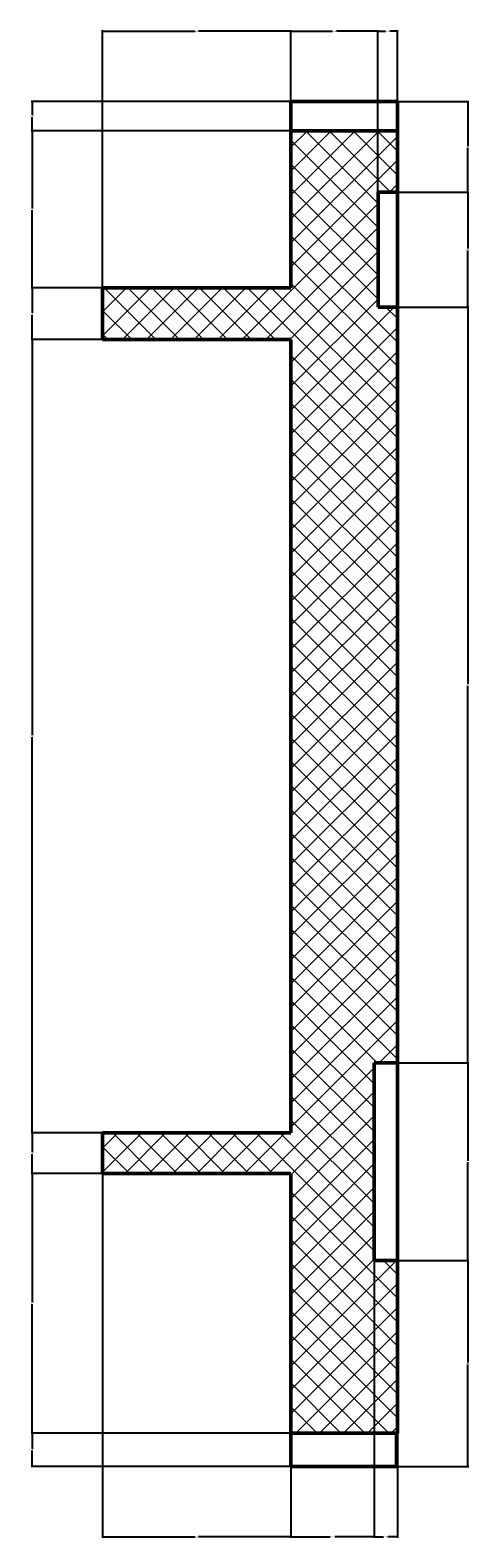
# Model space of a CAD drawing. Units: millimetres. Extents: x 2637 to 3282, y 1554 to 2264.
# Tile 3 of 3: x 3199 to 3282, y 1976 to 2260. Entities that reach past the tile are written whole.
import ezdxf

# ---------------------------------------------------------------- set-up
doc = ezdxf.new("R2010")
doc.units = ezdxf.units.MM
for name, color, linetype, lineweight in [('M-DIMS', 2, 'Continuous', 18), ('M-HATC', 8, 'Continuous', 18), ('M-OUTL', 7, 'Continuous', 50)]:
    doc.layers.add(name, color=color, linetype=linetype, lineweight=lineweight)
doc.styles.get("Standard").update_dxf_attribs({"font": 'arial.ttf'})
doc.dimstyles.get("Standard").update_dxf_attribs({"dimtxt": 0.18, "dimasz": 0.18, "dimexe": 0.18, "dimexo": 0.0625, "dimgap": 0.09, "dimtad": 0, "dimtih": 1, "dimtoh": 1, "dimdec": 4, "dimzin": 0, "dimdsep": 46, "dimtxsty": 'Standard', "dimcen": 0.09, "dimadec": 0, "dimazin": 0, "dimtfac": 1, "dimtdec": 4, "dimtofl": 0, "dimtmove": 0, "dimatfit": 3, "dimfxl": 1, "dimtolj": 1, "dimtzin": 0, "dimarcsym": 0})

# ---------------------------------------------------------------- blocks, each defined once
blk = doc.blocks.new('*D25')
at = {"layer": 'Defpoints', "color": 0, "transparency": 16777216}
for p in [(3247.95, 2259.5), (3212.55, 2211.25), (3247.95, 2211.25)]:
    blk.add_point(p, dxfattribs=at)
at = {"layer": 'M-DIMS', "color": 0, "lineweight": -2, "transparency": 16777216}
for p, q in [((3212.55, 2211.32), (3212.55, 2259.68)), ((3212.73, 2259.5), (3229.93, 2259.5)), ((3247.77, 2259.5), (3230.58, 2259.5)), ((3247.95, 2211.32), (3247.95, 2259.68))]:
    blk.add_line(p, q, dxfattribs=at)
at = {"layer": 'M-DIMS', "color": 0, "transparency": 16777216}
for points in [[(3212.73, 2259.53), (3212.73, 2259.47), (3212.55, 2259.5)], [(3247.77, 2259.53), (3247.77, 2259.47), (3247.95, 2259.5)]]:
    blk.add_solid(points, dxfattribs=at)
at = {"layer": 'M-DIMS', "color": 0, "transparency": 16777216, "insert": (3230.25, 2259.5), "char_height": 0.18, "attachment_point": 5}
blk.add_mtext('\\A1;35.4', dxfattribs=at)
blk = doc.blocks.new('*D26')
at = {"layer": 'Defpoints', "color": 0, "transparency": 16777216}
for p in [(3264.31, 2259.5), (3247.95, 2246.25), (3264.31, 2229.26)]:
    blk.add_point(p, dxfattribs=at)
at = {"layer": 'M-DIMS', "color": 0, "lineweight": -2, "transparency": 16777216}
for p, q in [((3247.95, 2246.31), (3247.95, 2259.68)), ((3248.13, 2259.5), (3255.75, 2259.5)), ((3264.13, 2259.5), (3256.52, 2259.5)), ((3264.31, 2229.32), (3264.31, 2259.68))]:
    blk.add_line(p, q, dxfattribs=at)
at = {"layer": 'M-DIMS', "color": 0, "transparency": 16777216}
for points in [[(3248.13, 2259.53), (3248.13, 2259.47), (3247.95, 2259.5)], [(3264.13, 2259.53), (3264.13, 2259.47), (3264.31, 2259.5)]]:
    blk.add_solid(points, dxfattribs=at)
at = {"layer": 'M-DIMS', "color": 0, "transparency": 16777216, "insert": (3256.13, 2259.5), "char_height": 0.18, "attachment_point": 5}
blk.add_mtext('\\A1;16.36', dxfattribs=at)
blk = doc.blocks.new('*D27')
at = {"layer": 'Defpoints', "color": 0, "transparency": 16777216}
for p in [(3267.95, 2259.5), (3264.31, 2229.26), (3267.95, 2229.26)]:
    blk.add_point(p, dxfattribs=at)
at = {"layer": 'M-DIMS', "color": 0, "lineweight": -2, "transparency": 16777216}
for p, q in [((3264.31, 2229.32), (3264.31, 2259.68)), ((3264.49, 2259.5), (3265.74, 2259.5)), ((3267.77, 2259.5), (3266.53, 2259.5)), ((3267.95, 2229.32), (3267.95, 2259.68))]:
    blk.add_line(p, q, dxfattribs=at)
at = {"layer": 'M-DIMS', "color": 0, "transparency": 16777216}
for points in [[(3264.49, 2259.53), (3264.49, 2259.47), (3264.31, 2259.5)], [(3267.77, 2259.53), (3267.77, 2259.47), (3267.95, 2259.5)]]:
    blk.add_solid(points, dxfattribs=at)
at = {"layer": 'M-DIMS', "color": 0, "transparency": 16777216, "insert": (3266.13, 2259.5), "char_height": 0.18, "attachment_point": 5}
blk.add_mtext('\\A1;3.639', dxfattribs=at)
blk = doc.blocks.new('*D28')
at = {"layer": 'Defpoints', "color": 0, "transparency": 16777216}
for p in [(3212.55, 2044.85), (3247.95, 2044.85), (3247.95, 1976.59)]:
    blk.add_point(p, dxfattribs=at)
at = {"layer": 'M-DIMS', "color": 0, "lineweight": -2, "transparency": 16777216}
for p, q in [((3212.55, 2044.79), (3212.55, 1976.41)), ((3247.95, 2044.79), (3247.95, 1976.41)), ((3212.73, 1976.59), (3229.93, 1976.59)), ((3247.77, 1976.59), (3230.58, 1976.59))]:
    blk.add_line(p, q, dxfattribs=at)
at = {"layer": 'M-DIMS', "color": 0, "transparency": 16777216}
for points in [[(3212.73, 1976.62), (3212.73, 1976.56), (3212.55, 1976.59)], [(3247.77, 1976.62), (3247.77, 1976.56), (3247.95, 1976.59)]]:
    blk.add_solid(points, dxfattribs=at)
at = {"layer": 'M-DIMS', "color": 0, "transparency": 16777216, "insert": (3230.25, 1976.59), "char_height": 0.18, "attachment_point": 5}
blk.add_mtext('\\A1;35.4', dxfattribs=at)
blk = doc.blocks.new('*D29')
at = {"layer": 'Defpoints', "color": 0, "transparency": 16777216}
for p in [(3263.56, 2028.52), (3247.95, 1989.84), (3263.56, 1976.59)]:
    blk.add_point(p, dxfattribs=at)
at = {"layer": 'M-DIMS', "color": 0, "lineweight": -2, "transparency": 16777216}
for p, q in [((3263.56, 2028.46), (3263.56, 1976.41)), ((3247.95, 1989.77), (3247.95, 1976.41)), ((3248.13, 1976.59), (3255.3, 1976.59)), ((3263.38, 1976.59), (3256.21, 1976.59))]:
    blk.add_line(p, q, dxfattribs=at)
at = {"layer": 'M-DIMS', "color": 0, "transparency": 16777216}
for points in [[(3248.13, 1976.62), (3248.13, 1976.56), (3247.95, 1976.59)], [(3263.38, 1976.62), (3263.38, 1976.56), (3263.56, 1976.59)]]:
    blk.add_solid(points, dxfattribs=at)
at = {"layer": 'M-DIMS', "color": 0, "transparency": 16777216, "insert": (3255.76, 1976.59), "char_height": 0.18, "attachment_point": 5}
blk.add_mtext('\\A1;15.612', dxfattribs=at)
blk = doc.blocks.new('*D30')
at = {"layer": 'Defpoints', "color": 0, "transparency": 16777216}
for p in [(3263.56, 2028.52), (3267.95, 2028.52), (3267.95, 1976.59)]:
    blk.add_point(p, dxfattribs=at)
at = {"layer": 'M-DIMS', "color": 0, "lineweight": -2, "transparency": 16777216}
for p, q in [((3263.56, 2028.46), (3263.56, 1976.41)), ((3267.95, 2028.46), (3267.95, 1976.41)), ((3263.74, 1976.59), (3265.36, 1976.59)), ((3267.77, 1976.59), (3266.15, 1976.59))]:
    blk.add_line(p, q, dxfattribs=at)
at = {"layer": 'M-DIMS', "color": 0, "transparency": 16777216}
for points in [[(3263.74, 1976.62), (3263.74, 1976.56), (3263.56, 1976.59)], [(3267.77, 1976.62), (3267.77, 1976.56), (3267.95, 1976.59)]]:
    blk.add_solid(points, dxfattribs=at)
at = {"layer": 'M-DIMS', "color": 0, "transparency": 16777216, "insert": (3265.76, 1976.59), "char_height": 0.18, "attachment_point": 5}
blk.add_mtext('\\A1;4.388', dxfattribs=at)
blk = doc.blocks.new('*D31')
at = {"layer": 'Defpoints', "color": 0, "transparency": 16777216}
for p in [(3247.95, 2246.25), (3199.3, 2240.76), (3247.95, 2240.76)]:
    blk.add_point(p, dxfattribs=at)
at = {"layer": 'M-DIMS', "color": 0, "lineweight": -2, "transparency": 16777216}
for p, q in [((3247.89, 2246.25), (3199.12, 2246.25)), ((3199.3, 2246.07), (3199.3, 2243.69)), ((3247.89, 2240.76), (3199.12, 2240.76)), ((3199.3, 2240.94), (3199.3, 2243.32))]:
    blk.add_line(p, q, dxfattribs=at)
at = {"layer": 'M-DIMS', "color": 0, "transparency": 16777216}
for points in [[(3199.27, 2246.07), (3199.33, 2246.07), (3199.3, 2246.25)], [(3199.27, 2240.94), (3199.33, 2240.94), (3199.3, 2240.76)]]:
    blk.add_solid(points, dxfattribs=at)
at = {"layer": 'M-DIMS', "color": 0, "transparency": 16777216, "insert": (3199.3, 2243.5), "char_height": 0.18, "attachment_point": 5}
blk.add_mtext('\\A1;5.483', dxfattribs=at)
blk = doc.blocks.new('*D32')
at = {"layer": 'Defpoints', "color": 0, "transparency": 16777216}
for p in [(3247.95, 2240.76), (3199.3, 2211.25), (3212.55, 2211.25)]:
    blk.add_point(p, dxfattribs=at)
at = {"layer": 'M-DIMS', "color": 0, "lineweight": -2, "transparency": 16777216}
for p, q in [((3247.89, 2240.76), (3199.12, 2240.76)), ((3199.3, 2240.58), (3199.3, 2226.19)), ((3199.3, 2211.43), (3199.3, 2225.83)), ((3212.49, 2211.25), (3199.12, 2211.25))]:
    blk.add_line(p, q, dxfattribs=at)
at = {"layer": 'M-DIMS', "color": 0, "transparency": 16777216}
for points in [[(3199.27, 2240.58), (3199.33, 2240.58), (3199.3, 2240.76)], [(3199.27, 2211.43), (3199.33, 2211.43), (3199.3, 2211.25)]]:
    blk.add_solid(points, dxfattribs=at)
at = {"layer": 'M-DIMS', "color": 0, "transparency": 16777216, "insert": (3199.3, 2226.01), "char_height": 0.18, "attachment_point": 5}
blk.add_mtext('\\A1;29.51', dxfattribs=at)
blk = doc.blocks.new('*D33')
at = {"layer": 'Defpoints', "color": 0, "transparency": 16777216}
for p in [(3212.55, 2211.25), (3199.3, 2201.55), (3212.55, 2201.55)]:
    blk.add_point(p, dxfattribs=at)
at = {"layer": 'M-DIMS', "color": 0, "lineweight": -2, "transparency": 16777216}
for p, q in [((3212.49, 2211.25), (3199.12, 2211.25)), ((3199.3, 2211.07), (3199.3, 2206.58)), ((3199.3, 2201.73), (3199.3, 2206.22)), ((3212.49, 2201.55), (3199.12, 2201.55))]:
    blk.add_line(p, q, dxfattribs=at)
at = {"layer": 'M-DIMS', "color": 0, "transparency": 16777216}
for points in [[(3199.27, 2211.07), (3199.33, 2211.07), (3199.3, 2211.25)], [(3199.27, 2201.73), (3199.33, 2201.73), (3199.3, 2201.55)]]:
    blk.add_solid(points, dxfattribs=at)
at = {"layer": 'M-DIMS', "color": 0, "transparency": 16777216, "insert": (3199.3, 2206.4), "char_height": 0.18, "attachment_point": 5}
blk.add_mtext('\\A1;9.707', dxfattribs=at)
blk = doc.blocks.new('*D34')
at = {"layer": 'Defpoints', "color": 0, "transparency": 16777216}
for p in [(3212.55, 2201.55), (3199.3, 2052.48), (3212.55, 2052.48)]:
    blk.add_point(p, dxfattribs=at)
at = {"layer": 'M-DIMS', "color": 0, "lineweight": -2, "transparency": 16777216}
for p, q in [((3212.49, 2201.55), (3199.12, 2201.55)), ((3199.3, 2201.37), (3199.3, 2127.19)), ((3199.3, 2052.66), (3199.3, 2126.83)), ((3212.49, 2052.48), (3199.12, 2052.48))]:
    blk.add_line(p, q, dxfattribs=at)
at = {"layer": 'M-DIMS', "color": 0, "transparency": 16777216}
for points in [[(3199.27, 2201.37), (3199.33, 2201.37), (3199.3, 2201.55)], [(3199.27, 2052.66), (3199.33, 2052.66), (3199.3, 2052.48)]]:
    blk.add_solid(points, dxfattribs=at)
at = {"layer": 'M-DIMS', "color": 0, "transparency": 16777216, "insert": (3199.3, 2127.01), "char_height": 0.18, "attachment_point": 5}
blk.add_mtext('\\A1;149.07', dxfattribs=at)
blk = doc.blocks.new('*D35')
at = {"layer": 'Defpoints', "color": 0, "transparency": 16777216}
for p in [(3212.55, 2052.48), (3199.3, 2044.85), (3212.55, 2044.85)]:
    blk.add_point(p, dxfattribs=at)
at = {"layer": 'M-DIMS', "color": 0, "lineweight": -2, "transparency": 16777216}
for p, q in [((3212.49, 2052.48), (3199.12, 2052.48)), ((3199.3, 2052.3), (3199.3, 2048.84)), ((3199.3, 2045.03), (3199.3, 2048.48)), ((3212.49, 2044.85), (3199.12, 2044.85))]:
    blk.add_line(p, q, dxfattribs=at)
at = {"layer": 'M-DIMS', "color": 0, "transparency": 16777216}
for points in [[(3199.27, 2052.3), (3199.33, 2052.3), (3199.3, 2052.48)], [(3199.27, 2045.03), (3199.33, 2045.03), (3199.3, 2044.85)]]:
    blk.add_solid(points, dxfattribs=at)
at = {"layer": 'M-DIMS', "color": 0, "transparency": 16777216, "insert": (3199.3, 2048.66), "char_height": 0.18, "attachment_point": 5}
blk.add_mtext('\\A1;7.627', dxfattribs=at)
blk = doc.blocks.new('*D36')
at = {"layer": 'Defpoints', "color": 0, "transparency": 16777216}
for p in [(3212.55, 2044.85), (3199.3, 1996.1), (3247.95, 1996.1)]:
    blk.add_point(p, dxfattribs=at)
at = {"layer": 'M-DIMS', "color": 0, "lineweight": -2, "transparency": 16777216}
for p, q in [((3212.49, 2044.85), (3199.12, 2044.85)), ((3199.3, 2044.67), (3199.3, 2020.66)), ((3199.3, 1996.28), (3199.3, 2020.29)), ((3247.89, 1996.1), (3199.12, 1996.1))]:
    blk.add_line(p, q, dxfattribs=at)
at = {"layer": 'M-DIMS', "color": 0, "transparency": 16777216}
for points in [[(3199.27, 2044.67), (3199.33, 2044.67), (3199.3, 2044.85)], [(3199.27, 1996.28), (3199.33, 1996.28), (3199.3, 1996.1)]]:
    blk.add_solid(points, dxfattribs=at)
at = {"layer": 'M-DIMS', "color": 0, "transparency": 16777216, "insert": (3199.3, 2020.48), "char_height": 0.18, "attachment_point": 5}
blk.add_mtext('\\A1;48.75', dxfattribs=at)
blk = doc.blocks.new('*D37')
at = {"layer": 'Defpoints', "color": 0, "transparency": 16777216}
for p in [(3247.95, 1996.1), (3199.3, 1989.84), (3247.95, 1989.84)]:
    blk.add_point(p, dxfattribs=at)
at = {"layer": 'M-DIMS', "color": 0, "lineweight": -2, "transparency": 16777216}
for p, q in [((3247.89, 1996.1), (3199.12, 1996.1)), ((3199.3, 1995.92), (3199.3, 1993.15)), ((3199.3, 1990.02), (3199.3, 1992.79)), ((3247.89, 1989.84), (3199.12, 1989.84))]:
    blk.add_line(p, q, dxfattribs=at)
at = {"layer": 'M-DIMS', "color": 0, "transparency": 16777216}
for points in [[(3199.27, 1995.92), (3199.33, 1995.92), (3199.3, 1996.1)], [(3199.27, 1990.02), (3199.33, 1990.02), (3199.3, 1989.84)]]:
    blk.add_solid(points, dxfattribs=at)
at = {"layer": 'M-DIMS', "color": 0, "transparency": 16777216, "insert": (3199.3, 1992.97), "char_height": 0.18, "attachment_point": 5}
blk.add_mtext('\\A1;6.267', dxfattribs=at)
blk = doc.blocks.new('*D38')
at = {"layer": 'Defpoints', "color": 0, "transparency": 16777216}
for p in [(3267.95, 2028.52), (3281.2, 2028.52), (3267.78, 1989.84)]:
    blk.add_point(p, dxfattribs=at)
at = {"layer": 'M-DIMS', "color": 0, "lineweight": -2, "transparency": 16777216}
for p, q in [((3268.01, 2028.52), (3281.38, 2028.52)), ((3281.2, 2028.34), (3281.2, 2009.36)), ((3281.2, 1990.02), (3281.2, 2009)), ((3267.84, 1989.84), (3281.38, 1989.84))]:
    blk.add_line(p, q, dxfattribs=at)
at = {"layer": 'M-DIMS', "color": 0, "transparency": 16777216}
for points in [[(3281.17, 2028.34), (3281.23, 2028.34), (3281.2, 2028.52)], [(3281.17, 1990.02), (3281.23, 1990.02), (3281.2, 1989.84)]]:
    blk.add_solid(points, dxfattribs=at)
at = {"layer": 'M-DIMS', "color": 0, "transparency": 16777216, "insert": (3281.2, 2009.18), "char_height": 0.18, "attachment_point": 5}
blk.add_mtext('\\A1;38.686', dxfattribs=at)
blk = doc.blocks.new('*D39')
at = {"layer": 'Defpoints', "color": 0, "transparency": 16777216}
for p in [(3267.95, 2065.64), (3281.2, 2065.64), (3267.95, 2028.52)]:
    blk.add_point(p, dxfattribs=at)
at = {"layer": 'M-DIMS', "color": 0, "lineweight": -2, "transparency": 16777216}
for p, q in [((3268.01, 2065.64), (3281.38, 2065.64)), ((3281.2, 2065.46), (3281.2, 2047.26)), ((3281.2, 2028.7), (3281.2, 2046.9)), ((3268.01, 2028.52), (3281.38, 2028.52))]:
    blk.add_line(p, q, dxfattribs=at)
at = {"layer": 'M-DIMS', "color": 0, "transparency": 16777216}
for points in [[(3281.17, 2065.46), (3281.23, 2065.46), (3281.2, 2065.64)], [(3281.17, 2028.7), (3281.23, 2028.7), (3281.2, 2028.52)]]:
    blk.add_solid(points, dxfattribs=at)
at = {"layer": 'M-DIMS', "color": 0, "transparency": 16777216, "insert": (3281.2, 2047.08), "char_height": 0.18, "attachment_point": 5}
blk.add_mtext('\\A1;37.12', dxfattribs=at)
blk = doc.blocks.new('*D40')
at = {"layer": 'Defpoints', "color": 0, "transparency": 16777216}
for p in [(3267.95, 2207.66), (3281.2, 2207.66), (3267.95, 2065.64)]:
    blk.add_point(p, dxfattribs=at)
at = {"layer": 'M-DIMS', "color": 0, "lineweight": -2, "transparency": 16777216}
for p, q in [((3268.01, 2207.66), (3281.38, 2207.66)), ((3281.2, 2207.48), (3281.2, 2136.83)), ((3281.2, 2065.82), (3281.2, 2136.47)), ((3268.01, 2065.64), (3281.38, 2065.64))]:
    blk.add_line(p, q, dxfattribs=at)
at = {"layer": 'M-DIMS', "color": 0, "transparency": 16777216}
for points in [[(3281.17, 2207.48), (3281.23, 2207.48), (3281.2, 2207.66)], [(3281.17, 2065.82), (3281.23, 2065.82), (3281.2, 2065.64)]]:
    blk.add_solid(points, dxfattribs=at)
at = {"layer": 'M-DIMS', "color": 0, "transparency": 16777216, "insert": (3281.2, 2136.65), "char_height": 0.18, "attachment_point": 5}
blk.add_mtext('\\A1;142.02', dxfattribs=at)
blk = doc.blocks.new('*D41')
at = {"layer": 'Defpoints', "color": 0, "transparency": 16777216}
for p in [(3267.95, 2229.26), (3281.2, 2229.26), (3267.95, 2207.66)]:
    blk.add_point(p, dxfattribs=at)
at = {"layer": 'M-DIMS', "color": 0, "lineweight": -2, "transparency": 16777216}
for p, q in [((3268.01, 2229.26), (3281.38, 2229.26)), ((3281.2, 2229.08), (3281.2, 2218.64)), ((3281.2, 2207.84), (3281.2, 2218.28)), ((3268.01, 2207.66), (3281.38, 2207.66))]:
    blk.add_line(p, q, dxfattribs=at)
at = {"layer": 'M-DIMS', "color": 0, "transparency": 16777216}
for points in [[(3281.17, 2229.08), (3281.23, 2229.08), (3281.2, 2229.26)], [(3281.17, 2207.84), (3281.23, 2207.84), (3281.2, 2207.66)]]:
    blk.add_solid(points, dxfattribs=at)
at = {"layer": 'M-DIMS', "color": 0, "transparency": 16777216, "insert": (3281.2, 2218.46), "char_height": 0.18, "attachment_point": 5}
blk.add_mtext('\\A1;21.596', dxfattribs=at)
blk = doc.blocks.new('*D42')
at = {"layer": 'Defpoints', "color": 0, "transparency": 16777216}
for p in [(3267.95, 2246.25), (3281.2, 2246.25), (3267.95, 2229.26)]:
    blk.add_point(p, dxfattribs=at)
at = {"layer": 'M-DIMS', "color": 0, "lineweight": -2, "transparency": 16777216}
for p, q in [((3268.01, 2246.25), (3281.38, 2246.25)), ((3281.2, 2246.07), (3281.2, 2237.93)), ((3281.2, 2229.44), (3281.2, 2237.57)), ((3268.01, 2229.26), (3281.38, 2229.26))]:
    blk.add_line(p, q, dxfattribs=at)
at = {"layer": 'M-DIMS', "color": 0, "transparency": 16777216}
for points in [[(3281.17, 2246.07), (3281.23, 2246.07), (3281.2, 2246.25)], [(3281.17, 2229.44), (3281.23, 2229.44), (3281.2, 2229.26)]]:
    blk.add_solid(points, dxfattribs=at)
at = {"layer": 'M-DIMS', "color": 0, "transparency": 16777216, "insert": (3281.2, 2237.75), "char_height": 0.18, "attachment_point": 5}
blk.add_mtext('\\A1;16.99', dxfattribs=at)

msp = doc.modelspace()

# ---------------------------------------------------------------- hatches: boundary and pattern name
at = {"layer": 'M-HATC'}
h = msp.add_hatch(dxfattribs=at)
h.set_pattern_fill('ANSI37', color=256)
h.paths.add_polyline_path([(3267.951, 2028.5225), (3263.5629, 2028.5225), (3263.5629, 2065.6423), (3267.951, 2065.6423), (3267.951, 2207.6593), (3264.312, 2207.6593), (3264.312, 2229.2553), (3267.951, 2229.2553), (3267.951, 2240.7627), (3247.951, 2240.7627), (3247.951, 2211.2546), (3212.5536, 2211.2546), (3212.5536, 2201.5476), (3247.951, 2201.5476), (3247.951, 2052.476), (3212.5536, 2052.476), (3212.5536, 2044.849), (3247.951, 2044.849), (3247.951, 1996.1037), (3267.951, 1996.1037)])

# ---------------------------------------------------------------- linework, layer by layer
at = {"layer": 'M-OUTL'}
for p, q in [((3247.951, 2240.7627), (3247.951, 2246.246)), ((3247.951, 2246.246), (3267.7395, 2246.246)), ((3267.7395, 2246.246), (3267.951, 2246.246)), ((3267.951, 2246.246), (3267.951, 2240.7627)), ((3247.951, 2240.7627), (3267.951, 2240.7627)), ((3247.951, 2211.2546), (3247.951, 2240.7627)), ((3267.951, 2240.7627), (3267.951, 1996.1037)), ((3267.951, 2229.2553), (3264.312, 2229.2553)), ((3264.312, 2229.2553), (3264.312, 2207.6593)), ((3212.5536, 2201.5476), (3212.5536, 2211.2546)), ((3212.5536, 2211.2546), (3247.951, 2211.2546)), ((3264.312, 2207.6593), (3267.951, 2207.6593)), ((3247.951, 2201.5476), (3212.5536, 2201.5476)), ((3247.951, 2052.476), (3247.951, 2201.5476)), ((3263.5629, 2028.5225), (3263.5629, 2065.6423)), ((3263.5629, 2065.6423), (3267.951, 2065.6423)), ((3212.5536, 2044.849), (3212.5536, 2052.476)), ((3212.5536, 2052.476), (3247.951, 2052.476)), ((3247.951, 2044.849), (3212.5536, 2044.849)), ((3247.951, 1996.1037), (3247.951, 2044.849)), ((3267.951, 2028.5225), (3263.5629, 2028.5225)), ((3267.951, 1996.1037), (3247.951, 1996.1037)), ((3247.951, 1996.1037), (3247.951, 1989.8369)), ((3267.7823, 1989.8369), (3267.7823, 1996.1037)), ((3247.951, 1989.8369), (3267.7823, 1989.8369))]:
    msp.add_line(p, q, dxfattribs=at)

# ---------------------------------------------------------------- dimensions: what is measured, and where the dimension line sits
at = {"layer": 'M-DIMS'}
for base, p1, p2, override, picture, middle in [((3247.951, 2259.496), (3212.5536, 2211.2546), (3247.951, 2211.2546), {"dimdec": 1, "dimlfac": 1, "dimrnd": 0, "dimzin": 0, "dimdsep": 46, "dimlunit": 2}, '*D25', (3230.2523, 2259.496)), ((3264.312, 2259.496), (3247.951, 2246.246), (3264.312, 2229.2553), {"dimdec": 2, "dimlfac": 1, "dimrnd": 0, "dimzin": 0, "dimdsep": 46, "dimlunit": 2}, '*D26', (3256.1315, 2259.496)), ((3267.951, 2259.496), (3264.312, 2229.2553), (3267.951, 2229.2553), {"dimdec": 3, "dimlfac": 1, "dimrnd": 0, "dimzin": 0, "dimdsep": 46, "dimlunit": 2}, '*D27', (3266.1315, 2259.496)), ((3247.951, 1976.5869), (3212.5536, 2044.849), (3247.951, 2044.849), {"dimdec": 1, "dimlfac": 1, "dimrnd": 0, "dimzin": 0, "dimdsep": 46, "dimlunit": 2}, '*D28', (3230.2523, 1976.5869)), ((3263.5629, 1976.5869), (3247.951, 1989.8369), (3263.5629, 2028.5225), {"dimdec": 3, "dimlfac": 1, "dimrnd": 0, "dimzin": 0, "dimdsep": 46, "dimlunit": 2}, '*D29', (3255.757, 1976.5869)), ((3267.951, 1976.5869), (3263.5629, 2028.5225), (3267.951, 2028.5225), {"dimdec": 3, "dimlfac": 1, "dimrnd": 0, "dimzin": 0, "dimdsep": 46, "dimlunit": 2}, '*D30', (3265.757, 1976.5869))]:
    dim = msp.add_linear_dim(base=base, p1=p1, p2=p2, dimstyle='Standard', override=override, dxfattribs=at)
    dim.commit()
    dim.dimension.update_dxf_attribs({"geometry": picture, "text_midpoint": middle})
for base, p1, p2, override, picture, middle in [((3199.3036, 2240.7627), (3247.951, 2246.246), (3247.951, 2240.7627), {"dimdec": 3, "dimlfac": 1, "dimrnd": 0, "dimzin": 0, "dimdsep": 46, "dimlunit": 2}, '*D31', (3199.3036, 2243.5044)), ((3281.2011, 2246.246), (3267.951, 2229.2553), (3267.951, 2246.246), {"dimdec": 2, "dimlfac": 1, "dimrnd": 0, "dimzin": 0, "dimdsep": 46, "dimlunit": 2}, '*D42', (3281.2011, 2237.7507)), ((3199.3036, 2211.2546), (3247.951, 2240.7627), (3212.5536, 2211.2546), {"dimdec": 2, "dimlfac": 1, "dimrnd": 0, "dimzin": 0, "dimdsep": 46, "dimlunit": 2}, '*D32', (3199.3036, 2226.0086)), ((3281.2011, 2229.2553), (3267.951, 2207.6593), (3267.951, 2229.2553), {"dimdec": 3, "dimlfac": 1, "dimrnd": 0, "dimzin": 0, "dimdsep": 46, "dimlunit": 2}, '*D41', (3281.2011, 2218.4573)), ((3199.3036, 2201.5476), (3212.5536, 2211.2546), (3212.5536, 2201.5476), {"dimdec": 3, "dimlfac": 1, "dimrnd": 0, "dimzin": 0, "dimdsep": 46, "dimlunit": 2}, '*D33', (3199.3036, 2206.4011)), ((3281.2011, 2207.6593), (3267.951, 2065.6423), (3267.951, 2207.6593), {"dimdec": 2, "dimlfac": 1, "dimrnd": 0, "dimzin": 0, "dimdsep": 46, "dimlunit": 2}, '*D40', (3281.2011, 2136.6508)), ((3199.3036, 2052.476), (3212.5536, 2201.5476), (3212.5536, 2052.476), {"dimdec": 2, "dimlfac": 1, "dimrnd": 0, "dimzin": 0, "dimdsep": 46, "dimlunit": 2}, '*D34', (3199.3036, 2127.0118)), ((3281.2011, 2065.6423), (3267.951, 2028.5225), (3267.951, 2065.6423), {"dimdec": 2, "dimlfac": 1, "dimrnd": 0, "dimzin": 0, "dimdsep": 46, "dimlunit": 2}, '*D39', (3281.2011, 2047.0824)), ((3199.3036, 2044.849), (3212.5536, 2052.476), (3212.5536, 2044.849), {"dimdec": 3, "dimlfac": 1, "dimrnd": 0, "dimzin": 0, "dimdsep": 46, "dimlunit": 2}, '*D35', (3199.3036, 2048.6625)), ((3199.3036, 1996.1037), (3212.5536, 2044.849), (3247.951, 1996.1037), {"dimdec": 2, "dimlfac": 1, "dimrnd": 0, "dimzin": 0, "dimdsep": 46, "dimlunit": 2}, '*D36', (3199.3036, 2020.4764)), ((3281.2011, 2028.5225), (3267.7823, 1989.8369), (3267.951, 2028.5225), {"dimdec": 3, "dimlfac": 1, "dimrnd": 0, "dimzin": 0, "dimdsep": 46, "dimlunit": 2}, '*D38', (3281.2011, 2009.1797)), ((3199.3036, 1989.8369), (3247.951, 1996.1037), (3247.951, 1989.8369), {"dimdec": 3, "dimlfac": 1, "dimrnd": 0, "dimzin": 0, "dimdsep": 46, "dimlunit": 2}, '*D37', (3199.3036, 1992.9703))]:
    dim = msp.add_linear_dim(base=base, p1=p1, p2=p2, angle=90, dimstyle='Standard', override=override, dxfattribs=at)
    dim.commit()
    dim.dimension.update_dxf_attribs({"geometry": picture, "text_midpoint": middle})

doc.saveas('drawing.dxf')
